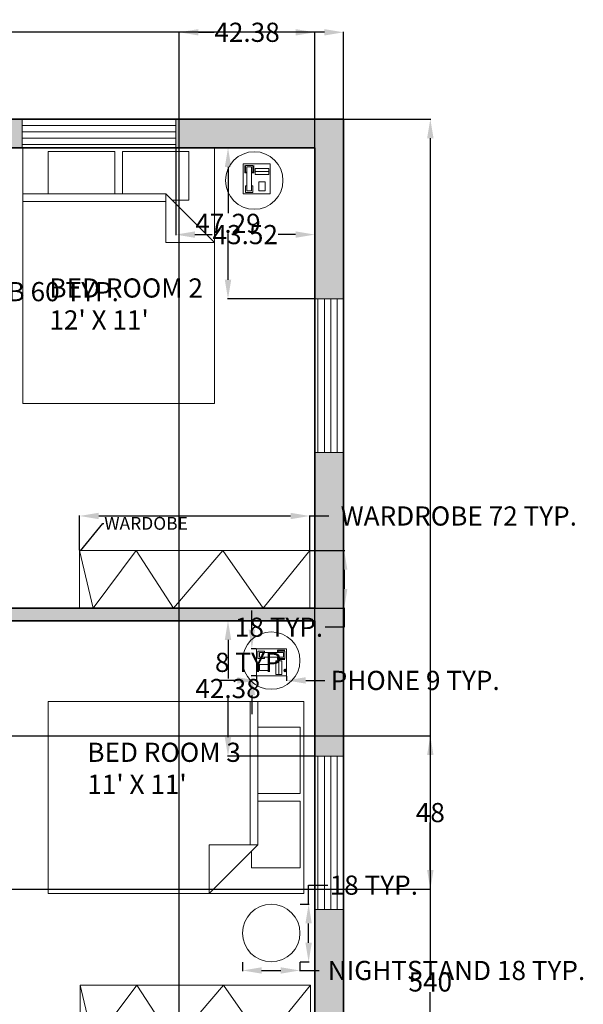
# Model space of a CAD drawing. Units: inches. Extents: x -16 to 578, y -553 to 49.
# Tile 5 of 5: x 402 to 578, y -259 to 49. Entities that reach past the tile are written whole.
import ezdxf
from ezdxf import colors
from ezdxf.entities.mleader import LeaderData, LeaderLine
from ezdxf.math import Vec2, Vec3

# ---------------------------------------------------------------- set-up
doc = ezdxf.new("R2010")
doc.units = ezdxf.units.IN
doc.header["$MEASUREMENT"] = 0
for name, color, linetype, lineweight in [('A-ANNO-DIMS', 2, 'Continuous', 18), ('A-ANNO-TEXT', 7, 'Continuous', 18), ('A-AREA-IDEN', 7, 'Continuous', 25), ('A-EQPM', 8, 'Continuous', 18), ('A-FLOR-CASE', 8, 'Continuous', 18), ('A-FURN', 8, 'Continuous', 18), ('A-GLAZ', 4, 'Continuous', 18), ('A-WALL', 7, 'Continuous', 35)]:
    doc.layers.add(name, color=color, linetype=linetype, lineweight=lineweight)
doc.layers.add('A-WALL-PATT', color=251, linetype='Continuous', lineweight=13, true_color=0x636466)
doc.styles.get("Standard").update_dxf_attribs({"font": 'arial.ttf'})
doc.dimstyles.get("Standard").update_dxf_attribs({"dimtxt": 6, "dimasz": 6, "dimexe": 0.18, "dimexo": 0.0625, "dimgap": 0.09, "dimtad": 0, "dimtih": 1, "dimtoh": 1, "dimdec": 0, "dimzin": 0, "dimdsep": 46, "dimlunit": 4, "dimtxsty": 'Standard', "dimcen": 0.09, "dimadec": 0, "dimazin": 0, "dimtfac": 1, "dimtdec": 0, "dimtofl": 0, "dimtmove": 0, "dimatfit": 3, "dimfxl": 1, "dimtolj": 1, "dimtzin": 0, "dimarcsym": 0})

# ---------------------------------------------------------------- blocks, each defined once
blk = doc.blocks.new('Bed - Queen')
for p, q in [((0, -80.00003), (0, 0)), ((0, 0), (59.99999, 0)), ((59.99999, 0), (59.99999, -80.00003)), ((7.99999, -1.2), (28.79998, -1.2)), ((7.99999, -14.4), (7.99999, -1.2)), ((28.79998, -1.2), (28.79998, -14.4)), ((31.19999, -1.2), (51.99999, -1.2)), ((31.19999, -14.4), (31.19999, -1.2)), ((51.99999, -1.2), (51.99999, -16.4)), ((0, -14.4), (44.8, -14.4)), ((59.99999, -29.6), (44.8, -14.4)), ((44.8, -14.4), (44.8, -29.6)), ((44.8, -16.8), (0, -16.8)), ((51.99999, -16.4), (46.79936, -16.4)), ((44.8, -29.6), (59.99999, -29.6)), ((59.99999, -80.00003), (0, -80.00003))]:
    blk.add_line(p, q)
blk = doc.blocks.new('Phone - Desk')
for p, q in [((-4.5, -5), (-4.5, 5)), ((-4.5, 5), (4.5, 5)), ((-4, 4.5), (-4, 2)), ((-3.75, 4.5), (-3.75, 2.25)), ((-1.25, 4.5), (-3.75, 4.5)), ((-3.25, 4), (-3.25, -4)), ((-3.25, 4), (-1.75, 4)), ((-1.75, -4), (-1.75, 4)), ((-1.25, 2.25), (-1.25, 4.5)), ((-1, 2), (-1, 4.5)), ((4, 3.5), (-0.5, 3.5)), ((-0.5, 3.5), (-0.5, 1.5)), ((4, 1.5), (4, 3.5)), ((4.5, 5), (4.5, -5)), ((-4, 2), (-3.25, 2)), ((-3.75, 2.25), (-3.25, 2.25)), ((-1.75, 2.25), (-1.25, 2.25)), ((-1.75, 2), (-1, 2)), ((-0.5, 2.5), (4, 2.5)), ((-0.5, 1.5), (4, 1.5)), ((-3.75, -2.25), (-3.25, -2.25)), ((-3.75, -4.5), (-3.75, -2.25)), ((-1.75, -2.25), (-1.25, -2.25)), ((-1.25, -2.25), (-1.25, -4.5)), ((2.75, -1), (0.75, -1)), ((0.75, -1), (0.75, -4)), ((2.75, -4), (2.75, -1)), ((4.5, -5), (-4.5, -5)), ((-1.25, -4.5), (-3.75, -4.5)), ((-3.25, -4), (-1.75, -4)), ((0.75, -4), (2.75, -4))]:
    blk.add_line(p, q)
blk = doc.blocks.new('WIN-48X9')
for p, q in [((-48, -4), (0, -4)), ((-48, -6), (0, -6)), ((-48, -8), (0, -8))]:
    blk.add_line(p, q)
for points in [[(0, 0), (0, -9), (-48, -9), (-48, 0)], [(-48, -2), (0, -2)]]:
    blk.add_lwpolyline(points, close=True)
blk = doc.blocks.new('WARDROBE-72X18')
for p, q in [((0, 0), (18, -14.58)), ((18, -14.58), (0, -27.16)), ((0, -27.16), (18, -42.59)), ((18, -42.59), (0, -54.31)), ((0, -54.31), (18, -67.75)), ((18, -67.75), (0, -72))]:
    blk.add_line(p, q)
blk.add_lwpolyline([(0, 0), (18, 0), (18, -72), (0, -72)], close=True)
blk = doc.blocks.new('NIGHTSTAND-ROUND-18')
blk.add_circle((0, 0), 9)
blk = doc.blocks.new('*D28')
at = {"layer": 'A-ANNO-DIMS', "color": 0, "lineweight": -2, "transparency": 16777216}
for p, q in [((471.56, -245.54), (471.56, -248.36)), ((489.56, -245.54), (489.56, -248.36)), ((477.56, -248.18), (483.56, -248.18)), ((489.56, -248.18), (495.56, -248.18))]:
    blk.add_line(p, q, dxfattribs=at)
at = {"layer": 'A-ANNO-DIMS', "color": 0, "transparency": 16777216}
for points in [[(477.56, -247.18), (477.56, -249.18), (471.56, -248.18)], [(483.56, -247.18), (483.56, -249.18), (489.56, -248.18)]]:
    blk.add_solid(points, dxfattribs=at)
at = {"layer": 'Defpoints', "color": 0, "transparency": 16777216}
for p in [(471.56, -245.48), (489.56, -245.48), (489.56, -248.18)]:
    blk.add_point(p, dxfattribs=at)
at = {"layer": 'A-ANNO-DIMS', "color": 0, "transparency": 16777216, "insert": (538.51, -248.18), "char_height": 6, "attachment_point": 5}
blk.add_mtext('\\A1;NIGHTSTAND 18 TYP.', dxfattribs=at)
blk = doc.blocks.new('*D29')
at = {"layer": 'A-ANNO-DIMS', "color": 0, "lineweight": -2, "transparency": 16777216}
for p, q in [((492.26, -227.48), (492.26, -221.48)), ((492.26, -221.48), (498.26, -221.48)), ((489.62, -227.48), (492.44, -227.48)), ((492.26, -239.48), (492.26, -233.48)), ((489.62, -245.48), (492.44, -245.48))]:
    blk.add_line(p, q, dxfattribs=at)
at = {"layer": 'A-ANNO-DIMS', "color": 0, "transparency": 16777216}
for points in [[(491.26, -233.48), (493.26, -233.48), (492.26, -227.48)], [(491.26, -239.48), (493.26, -239.48), (492.26, -245.48)]]:
    blk.add_solid(points, dxfattribs=at)
at = {"layer": 'Defpoints', "color": 0, "transparency": 16777216}
for p in [(489.56, -227.48), (492.26, -227.48), (489.56, -245.48)]:
    blk.add_point(p, dxfattribs=at)
at = {"layer": 'A-ANNO-DIMS', "color": 0, "transparency": 16777216, "insert": (512.67, -221.48), "char_height": 6, "attachment_point": 5}
blk.add_mtext('\\A1;18 TYP.', dxfattribs=at)
blk = doc.blocks.new('*D30')
at = {"layer": 'A-ANNO-DIMS', "color": 0, "lineweight": -2, "transparency": 16777216}
for p, q in [((420.6, -116.7), (420.6, -105.79)), ((426.6, -105.97), (486.6, -105.97)), ((492.6, -116.7), (492.6, -105.79)), ((492.6, -105.97), (498.6, -105.97))]:
    blk.add_line(p, q, dxfattribs=at)
at = {"layer": 'A-ANNO-DIMS', "color": 0, "transparency": 16777216}
for points in [[(426.6, -104.97), (426.6, -106.97), (420.6, -105.97)], [(486.6, -104.97), (486.6, -106.97), (492.6, -105.97)]]:
    blk.add_solid(points, dxfattribs=at)
at = {"layer": 'Defpoints', "color": 0, "transparency": 16777216}
for p in [(492.6, -105.97), (420.6, -116.77), (492.6, -116.77)]:
    blk.add_point(p, dxfattribs=at)
at = {"layer": 'A-ANNO-DIMS', "color": 0, "transparency": 16777216, "insert": (539.26, -105.97), "char_height": 6, "attachment_point": 5}
blk.add_mtext('\\A1;WARDROBE 72 TYP.', dxfattribs=at)
blk = doc.blocks.new('*D31')
at = {"layer": 'A-ANNO-DIMS', "color": 0, "lineweight": -2, "transparency": 16777216}
for p, q in [((492.66, -116.77), (503.58, -116.77)), ((503.4, -122.77), (503.4, -128.77)), ((492.66, -134.77), (503.58, -134.77)), ((503.4, -134.77), (503.4, -140.77)), ((503.4, -140.77), (497.4, -140.77))]:
    blk.add_line(p, q, dxfattribs=at)
at = {"layer": 'A-ANNO-DIMS', "color": 0, "transparency": 16777216}
for points in [[(502.4, -122.77), (504.4, -122.77), (503.4, -116.77)], [(502.4, -128.77), (504.4, -128.77), (503.4, -134.77)]]:
    blk.add_solid(points, dxfattribs=at)
at = {"layer": 'Defpoints', "color": 0, "transparency": 16777216}
for p in [(492.6, -116.77), (492.6, -134.77), (503.4, -134.77)]:
    blk.add_point(p, dxfattribs=at)
at = {"layer": 'A-ANNO-DIMS', "color": 0, "transparency": 16777216, "insert": (482.99, -140.77), "char_height": 6, "attachment_point": 5}
blk.add_mtext('\\A1;18 TYP.', dxfattribs=at)
blk = doc.blocks.new('*D34')
at = {"layer": 'A-ANNO-DIMS', "color": 0, "lineweight": -2, "transparency": 16777216}
for p, q in [((475.91, -156.07), (475.91, -157.6)), ((485.34, -156.07), (485.34, -157.6)), ((469.91, -157.42), (463.91, -157.42)), ((491.34, -157.42), (497.34, -157.42))]:
    blk.add_line(p, q, dxfattribs=at)
at = {"layer": 'A-ANNO-DIMS', "color": 0, "transparency": 16777216}
for points in [[(469.91, -156.42), (469.91, -158.42), (475.91, -157.42)], [(491.34, -156.42), (491.34, -158.42), (485.34, -157.42)]]:
    blk.add_solid(points, dxfattribs=at)
at = {"layer": 'Defpoints', "color": 0, "transparency": 16777216}
for p in [(475.91, -156.01), (485.34, -156.01), (485.34, -157.42)]:
    blk.add_point(p, dxfattribs=at)
at = {"layer": 'A-ANNO-DIMS', "color": 0, "transparency": 16777216, "insert": (525.62, -157.42), "char_height": 6, "attachment_point": 5}
blk.add_mtext('\\A1;PHONE 9 TYP.', dxfattribs=at)
blk = doc.blocks.new('*D35')
at = {"layer": 'A-ANNO-DIMS', "color": 0, "lineweight": -2, "transparency": 16777216}
for p, q in [((474.5, -141.53), (474.5, -135.53)), ((475.85, -147.53), (474.32, -147.53)), ((475.85, -156.01), (474.32, -156.01)), ((474.5, -162.01), (474.5, -168.01))]:
    blk.add_line(p, q, dxfattribs=at)
at = {"layer": 'A-ANNO-DIMS', "color": 0, "transparency": 16777216}
for points in [[(473.5, -141.53), (475.5, -141.53), (474.5, -147.53)], [(473.5, -162.01), (475.5, -162.01), (474.5, -156.01)]]:
    blk.add_solid(points, dxfattribs=at)
at = {"layer": 'Defpoints', "color": 0, "transparency": 16777216}
for p in [(475.91, -147.53), (474.5, -156.01), (475.91, -156.01)]:
    blk.add_point(p, dxfattribs=at)
at = {"layer": 'A-ANNO-DIMS', "color": 0, "transparency": 16777216, "insert": (474.5, -151.77), "char_height": 6, "attachment_point": 5}
blk.add_mtext('\\A1;8 TYP.', dxfattribs=at)
blk = doc.blocks.new('*D40')
at = {"layer": 'A-ANNO-DIMS', "color": 0, "lineweight": -2, "transparency": 16777216}
for p, q in [((298.19, -26.83), (298.19, -35.95)), ((358.19, -26.83), (358.19, -35.95)), ((304.19, -35.77), (352.19, -35.77)), ((358.19, -35.77), (364.19, -35.77))]:
    blk.add_line(p, q, dxfattribs=at)
at = {"layer": 'A-ANNO-DIMS', "color": 0, "transparency": 16777216}
for points in [[(304.19, -34.77), (304.19, -36.77), (298.19, -35.77)], [(352.19, -34.77), (352.19, -36.77), (358.19, -35.77)]]:
    blk.add_solid(points, dxfattribs=at)
at = {"layer": 'Defpoints', "color": 0, "transparency": 16777216}
for p in [(298.19, -26.77), (358.19, -26.77), (358.19, -35.77)]:
    blk.add_point(p, dxfattribs=at)
at = {"layer": 'A-ANNO-DIMS', "color": 0, "transparency": 16777216, "insert": (399.47, -35.77), "char_height": 6, "attachment_point": 5}
blk.add_mtext('\\A1;BATHTUB 60 TYP.', dxfattribs=at)
blk = doc.blocks.new('*D62')
at = {"layer": 'A-ANNO-DIMS', "color": 0, "lineweight": -2, "transparency": 16777216}
for p, q in [((23.19, 18.3), (23.19, 45.56)), ((29.19, 45.38), (256.36, 45.38)), ((497.19, 45.38), (270.02, 45.38)), ((503.19, 18.3), (503.19, 45.56))]:
    blk.add_line(p, q, dxfattribs=at)
at = {"layer": 'A-ANNO-DIMS', "color": 0, "transparency": 16777216}
for points in [[(29.19, 46.38), (29.19, 44.38), (23.19, 45.38)], [(497.19, 46.38), (497.19, 44.38), (503.19, 45.38)]]:
    blk.add_solid(points, dxfattribs=at)
at = {"layer": 'Defpoints', "color": 0, "transparency": 16777216}
for p in [(503.19, 45.38), (23.19, 18.23), (503.19, 18.23)]:
    blk.add_point(p, dxfattribs=at)
at = {"layer": 'A-ANNO-DIMS', "color": 0, "transparency": 16777216, "insert": (263.19, 45.38), "char_height": 6, "attachment_point": 5}
blk.add_mtext('\\A1;480', dxfattribs=at)
blk = doc.blocks.new('*D63')
at = {"layer": 'A-ANNO-DIMS', "color": 0, "lineweight": -2, "transparency": 16777216}
for p, q in [((503.25, 18.23), (530.52, 18.23)), ((530.34, 12.23), (530.34, -248.61)), ((530.34, -515.77), (530.34, -254.92)), ((503.25, -521.77), (530.52, -521.77))]:
    blk.add_line(p, q, dxfattribs=at)
at = {"layer": 'A-ANNO-DIMS', "color": 0, "transparency": 16777216}
for points in [[(529.34, 12.23), (531.34, 12.23), (530.34, 18.23)], [(529.34, -515.77), (531.34, -515.77), (530.34, -521.77)]]:
    blk.add_solid(points, dxfattribs=at)
at = {"layer": 'Defpoints', "color": 0, "transparency": 16777216}
for p in [(503.19, 18.23), (503.19, -521.77), (530.34, -521.77)]:
    blk.add_point(p, dxfattribs=at)
at = {"layer": 'A-ANNO-DIMS', "color": 0, "transparency": 16777216, "insert": (530.34, -251.77), "char_height": 6, "attachment_point": 5}
blk.add_mtext('\\A1;540', dxfattribs=at)
blk = doc.blocks.new('*D69')
at = {"layer": 'A-ANNO-DIMS', "color": 0, "lineweight": -2, "transparency": 16777216}
for p, q in [((168.25, -174.77), (530.52, -174.77)), ((530.34, -180.77), (530.34, -195.61)), ((530.34, -216.77), (530.34, -201.92)), ((168.25, -222.77), (530.52, -222.77))]:
    blk.add_line(p, q, dxfattribs=at)
at = {"layer": 'A-ANNO-DIMS', "color": 0, "transparency": 16777216}
for points in [[(529.34, -180.77), (531.34, -180.77), (530.34, -174.77)], [(529.34, -216.77), (531.34, -216.77), (530.34, -222.77)]]:
    blk.add_solid(points, dxfattribs=at)
at = {"layer": 'Defpoints', "color": 0, "transparency": 16777216}
for p in [(168.19, -174.77), (168.19, -222.77), (530.34, -222.77)]:
    blk.add_point(p, dxfattribs=at)
at = {"layer": 'A-ANNO-DIMS', "color": 0, "transparency": 16777216, "insert": (530.34, -198.77), "char_height": 6, "attachment_point": 5}
blk.add_mtext('\\A1;48', dxfattribs=at)
blk = doc.blocks.new('*D74')
at = {"layer": 'A-ANNO-DIMS', "color": 0, "lineweight": -2, "transparency": 16777216}
for p, q in [((450.67, 9.17), (450.67, -18.1)), ((494.19, 9.17), (494.19, -18.1)), ((456.67, -17.92), (462.13, -17.92)), ((488.19, -17.92), (482.73, -17.92))]:
    blk.add_line(p, q, dxfattribs=at)
at = {"layer": 'A-ANNO-DIMS', "color": 0, "transparency": 16777216}
for points in [[(456.67, -16.92), (456.67, -18.92), (450.67, -17.92)], [(488.19, -16.92), (488.19, -18.92), (494.19, -17.92)]]:
    blk.add_solid(points, dxfattribs=at)
at = {"layer": 'Defpoints', "color": 0, "transparency": 16777216}
for p in [(450.67, 9.23), (494.19, 9.23), (450.67, -17.92)]:
    blk.add_point(p, dxfattribs=at)
at = {"layer": 'A-ANNO-DIMS', "color": 0, "transparency": 16777216, "insert": (472.43, -17.92), "char_height": 6, "attachment_point": 5}
blk.add_mtext('\\A1;43.52', dxfattribs=at)
blk = doc.blocks.new('*D75')
at = {"layer": 'A-ANNO-DIMS', "color": 0, "lineweight": -2, "transparency": 16777216}
for p, q in [((494.13, 9.23), (466.86, 9.23)), ((467.04, 3.23), (467.04, -11.26)), ((467.04, -32.05), (467.04, -17.56)), ((494.13, -38.05), (466.86, -38.05))]:
    blk.add_line(p, q, dxfattribs=at)
at = {"layer": 'A-ANNO-DIMS', "color": 0, "transparency": 16777216}
for points in [[(466.04, 3.23), (468.04, 3.23), (467.04, 9.23)], [(466.04, -32.05), (468.04, -32.05), (467.04, -38.05)]]:
    blk.add_solid(points, dxfattribs=at)
at = {"layer": 'Defpoints', "color": 0, "transparency": 16777216}
for p in [(467.04, 9.23), (494.19, 9.23), (494.19, -38.05)]:
    blk.add_point(p, dxfattribs=at)
at = {"layer": 'A-ANNO-DIMS', "color": 0, "transparency": 16777216, "insert": (467.04, -14.41), "char_height": 6, "attachment_point": 5}
blk.add_mtext('\\A1;47.29', dxfattribs=at)
blk = doc.blocks.new('*D76')
at = {"layer": 'A-ANNO-DIMS', "color": 0, "lineweight": -2, "transparency": 16777216}
for p, q in [((494.13, -138.77), (466.86, -138.77)), ((467.04, -144.77), (467.04, -156.8)), ((467.04, -175.15), (467.04, -163.11)), ((494.13, -181.15), (466.86, -181.15))]:
    blk.add_line(p, q, dxfattribs=at)
at = {"layer": 'A-ANNO-DIMS', "color": 0, "transparency": 16777216}
for points in [[(466.04, -144.77), (468.04, -144.77), (467.04, -138.77)], [(466.04, -175.15), (468.04, -175.15), (467.04, -181.15)]]:
    blk.add_solid(points, dxfattribs=at)
at = {"layer": 'Defpoints', "color": 0, "transparency": 16777216}
for p in [(467.04, -138.77), (494.19, -138.77), (494.19, -181.15)]:
    blk.add_point(p, dxfattribs=at)
at = {"layer": 'A-ANNO-DIMS', "color": 0, "transparency": 16777216, "insert": (467.04, -159.96), "char_height": 6, "attachment_point": 5}
blk.add_mtext('\\A1;42.38', dxfattribs=at)
blk = doc.blocks.new('*D80')
at = {"layer": 'A-ANNO-DIMS', "color": 0, "lineweight": -2, "transparency": 16777216}
for p, q in [((451.8, -512.7), (451.8, 45.56)), ((457.8, 45.38), (462.66, 45.38)), ((488.19, 45.38), (483.34, 45.38)), ((494.19, -512.7), (494.19, 45.56))]:
    blk.add_line(p, q, dxfattribs=at)
at = {"layer": 'A-ANNO-DIMS', "color": 0, "transparency": 16777216}
for points in [[(457.8, 46.38), (457.8, 44.38), (451.8, 45.38)], [(488.19, 46.38), (488.19, 44.38), (494.19, 45.38)]]:
    blk.add_solid(points, dxfattribs=at)
at = {"layer": 'Defpoints', "color": 0, "transparency": 16777216}
for p in [(451.8, 45.38), (451.8, -512.77), (494.19, -512.77)]:
    blk.add_point(p, dxfattribs=at)
at = {"layer": 'A-ANNO-DIMS', "color": 0, "transparency": 16777216, "insert": (473, 45.38), "char_height": 6, "attachment_point": 5}
blk.add_mtext('\\A1;42.38', dxfattribs=at)

msp = doc.modelspace()

# ---------------------------------------------------------------- hatches: boundary and pattern name
at = {"layer": 'A-WALL-PATT'}
h = msp.add_hatch(color=256, dxfattribs=at)
h.dxf.hatch_style = 1
h.paths.add_polyline_path([(32.1882, 9.2337), (89.8211, 9.2337), (89.8211, 18.2337), (23.1882, 18.2337), (23.1882, -55.5259), (32.1882, -55.5259)])
h.paths.add_polyline_path([(219.6411, 18.2337), (137.8211, 18.2337), (137.8211, 9.2337), (146.4179, 9.2337), (188.1882, 9.2337), (188.1882, -98.7663), (192.1882, -98.7663), (192.1882, -72.7663), (238.1882, -72.7663), (238.1882, -68.7663), (192.1882, -68.7663), (192.1882, 9.2337), (219.6411, 9.2337)])
h.paths.add_polyline_path([(307.3924, 18.2337), (243.6411, 18.2337), (243.6411, 9.2337), (274.1882, 9.2337), (274.1882, -26.7663), (274.1882, -68.7663), (268.1882, -68.7663), (268.1882, -72.7663), (274.1882, -72.7663), (274.1882, -98.7663), (250.1882, -98.7663), (250.1882, -102.7663), (274.1882, -102.7663), (278.1882, -102.7663), (302.188, -102.8481), (302.188, -98.8481), (278.1882, -98.7663), (278.1882, -86.8559, -0.01827889), (278.1882, -85.7663), (278.1882, -72.7663), (284.1882, -72.7663), (284.1882, -68.7663), (278.1882, -68.7663), (278.1882, 9.2337), (307.3924, 9.2337)])
h.paths.add_polyline_path([(402.6701, 18.2337), (331.3924, 18.2337), (331.3924, 9.2337), (358.1882, 9.2337), (358.1882, -26.7663), (358.1882, -68.7663), (314.1882, -68.7663), (314.1882, -72.7663), (358.1882, -72.7663), (358.1882, -98.7663), (362.1882, -98.7663), (362.1882, 9.2337), (402.6701, 9.2337)])
h.paths.add_polyline_path([(503.1882, 18.2337), (450.6701, 18.2337), (450.6701, 9.2337), (462.8072, 9.2337), (494.1882, 9.2337), (494.1882, -38.053), (503.1882, -38.053)])
h.paths.add_polyline_path([(503.1882, -86.053), (494.1882, -86.053), (494.1882, -134.7663), (362.1882, -134.7663), (362.1882, -128.7663), (358.1882, -128.7663), (358.1882, -138.7663), (358.1882, -234.7663), (362.1882, -234.7663), (362.1882, -138.7663), (494.1882, -138.7663), (494.1882, -181.1501), (503.1882, -181.1501)])
h.paths.add_polyline_path([(503.1882, -229.1501), (494.1882, -229.1501), (494.1882, -270.7663), (362.1882, -270.7663), (362.1882, -264.7663), (358.1882, -264.7663), (358.1882, -294.7663), (358.1882, -323.1753), (362.1882, -323.1753), (362.1882, -298.7663), (362.1882, -294.7663), (362.1882, -274.7663), (494.1882, -274.7663), (494.1882, -294.7663), (494.1882, -298.7663), (494.1882, -310.411), (503.1882, -310.411)])
h.paths.add_polyline_path([(503.1882, -358.411), (494.1882, -358.411), (494.1882, -394.7663), (362.1882, -394.7663), (362.1882, -353.1753), (358.1882, -353.1753), (358.1882, -398.7663), (494.1882, -398.7663), (494.1882, -512.7663), (451.8049, -512.7663), (451.8049, -521.7663), (503.1882, -521.7663)])
h.paths.add_polyline_path([(403.8049, -512.7663), (176.1882, -512.7663), (176.1882, -441.7663), (172.1882, -441.7663), (172.1882, -512.7663), (150.1882, -512.7663), (150.1882, -521.7663), (403.8049, -521.7663)])
h.paths.add_polyline_path([(176.1882, -258.7663), (168.1882, -258.7663), (168.1882, -246.7663), (168.1882, -234.7663), (168.1882, -222.7663), (164.1882, -222.7663), (164.1882, -234.7663), (164.1882, -258.7663), (102.0641, -258.7663), (102.0641, -262.7663), (168.1882, -262.7663), (172.1882, -262.7663), (172.1882, -333.7663), (176.1882, -333.7663), (176.1882, -262.7663)])
h.paths.add_polyline_path([(32.1882, -262.7663), (54.0641, -262.7663), (54.0641, -258.7663), (32.1882, -258.7663), (32.1882, -229.1501), (23.1882, -229.1501), (23.1882, -283.4909), (23.1882, -470.2771), (32.1882, -470.2771), (32.1882, -283.4909)])
h.paths.add_polyline_path([(32.1882, -103.5259), (23.1882, -103.5259), (23.1882, -181.1501), (32.1882, -181.1501)])
h.paths.add_polyline_path([(192.1882, -128.7663), (188.1882, -128.7663), (188.1882, -134.7663), (32.1882, -134.7663), (32.1882, -138.7663), (164.1882, -138.7663), (164.1882, -162.7663), (164.1882, -174.7663), (168.1882, -174.7663), (168.1882, -162.7663), (168.1882, -138.7663), (192.1882, -138.7663)])

# ---------------------------------------------------------------- linework, layer by layer
at = {"layer": 'A-WALL'}
for p, q in [((362.1882, 9.2337), (494.1882, 9.2337)), ((494.1882, 9.2337), (494.1882, -134.7663)), ((362.1882, -134.7663), (494.1882, -134.7663)), ((362.1882, -138.7663), (494.1882, -138.7663)), ((494.1882, -138.7663), (494.1882, -270.7663))]:
    msp.add_line(p, q, dxfattribs=at)
msp.add_lwpolyline([(23.1882, -283.4909), (23.1882, 18.2337), (503.1882, 18.2337), (503.1882, -521.7663), (150.1882, -521.7663)], dxfattribs=at)

# ---------------------------------------------------------------- block references
at = {"layer": 'A-EQPM', "xscale": 0.9424999999999881, "yscale": 0.9424999999999881, "zscale": 0.9424999999999881}
msp.add_blockref('Phone - Desk', (476.0241, -0.4929), dxfattribs=at)
at = {"layer": 'A-EQPM', "xscale": 0.9424999999999881, "yscale": 0.9424999999999881, "zscale": 0.9424999999999881, "rotation": 270}
msp.add_blockref('Phone - Desk', (480.6266, -151.7679), dxfattribs=at)
at = {"layer": 'A-FLOR-CASE'}
for p, rotation in [((492.5998, -116.7663), 270), ((492.8002, -252.7663), 270.0000000000002)]:
    msp.add_blockref('WARDROBE-72X18', p, dxfattribs=dict(at, rotation=rotation))
at = {"layer": 'A-FURN'}
for name, p in [('Bed - Queen', (402.8072, 9.2337)), ('NIGHTSTAND-ROUND-18', (475.2432, -0.9972)), ('NIGHTSTAND-ROUND-18', (480.5554, -151.2068)), ('NIGHTSTAND-ROUND-18', (480.5554, -236.4807))]:
    msp.add_blockref(name, p, dxfattribs=at)
at = {"layer": 'A-FURN', "rotation": 270}
msp.add_blockref('Bed - Queen', (490.7863, -164.0447), dxfattribs=at)
at = {"layer": 'A-GLAZ'}
msp.add_blockref('WIN-48X9', (450.6701, 18.2337), dxfattribs=at)
for p, rotation in [((503.1882, -86.053), 270.0000000000001), ((503.1882, -229.1501), 270.0000000000002)]:
    msp.add_blockref('WIN-48X9', p, dxfattribs=dict(at, rotation=rotation))

# ---------------------------------------------------------------- texts
at = {"layer": 'A-AREA-IDEN', "char_height": 6, "attachment_point": 1}
for s, width, insert in [("BED ROOM 2\\P12' X 11'", 72.589877, (411.1588, -31.6281)), ("BED ROOM 3\\P11' X 11'", 82.456452, (423.0299, -176.9071))]:
    msp.add_mtext_dynamic_manual_height_columns(s, width=width, gutter_width=1, heights=[0], dxfattribs=dict(at, insert=insert))

# ---------------------------------------------------------------- dimensions: what is measured, and where the dimension line sits
at = {"layer": 'A-ANNO-DIMS'}
for base, p1, p2, override, picture, middle in [((503.1882, 45.3837), (23.1882, 18.2337), (503.1882, 18.2337), {"dimdec": 0, "dimlfac": 1, "dimrnd": 0, "dimzin": 0, "dimdsep": 46, "dimlunit": 2}, '*D62', (263.1882, 45.3837)), ((451.8049, 45.3837), (494.1882, -512.7663), (451.8049, -512.7663), {"dimdec": 2, "dimlfac": 1, "dimrnd": 0, "dimzin": 0, "dimdsep": 46, "dimlunit": 2}, '*D80', (472.9965, 45.3837))]:
    dim = msp.add_linear_dim(base=base, p1=p1, p2=p2, dimstyle='Standard', override=override, dxfattribs=at)
    dim.commit()
    dim.dimension.update_dxf_attribs({"geometry": picture, "text_midpoint": middle})
for base, p1, p2, angle, override, picture, middle in [((530.3382, -521.7663), (503.1882, 18.2337), (503.1882, -521.7663), 90, {"dimdec": 0, "dimlfac": 1, "dimrnd": 0, "dimzin": 0, "dimdsep": 46, "dimlunit": 2}, '*D63', (530.3382, -251.7663)), ((450.6701, -17.9163), (494.1882, 9.2337), (450.6701, 9.2337), 180, {"dimdec": 2, "dimlfac": 1, "dimrnd": 0, "dimzin": 0, "dimdsep": 46, "dimlunit": 2}, '*D74', (472.4291, -17.9163)), ((467.0382, 9.2337), (494.1882, -38.053), (494.1882, 9.2337), 90, {"dimdec": 2, "dimlfac": 1, "dimrnd": 0, "dimzin": 0, "dimdsep": 46, "dimlunit": 2}, '*D75', (467.0382, -14.4096)), ((467.0382, -138.7663), (494.1882, -181.1501), (494.1882, -138.7663), 90, {"dimdec": 2, "dimlfac": 1, "dimrnd": 0, "dimzin": 0, "dimdsep": 46, "dimlunit": 2}, '*D76', (467.0382, -159.9582)), ((530.3382, -222.7663), (168.1882, -174.7663), (168.1882, -222.7663), 90, {"dimdec": 0, "dimlfac": 1, "dimrnd": 0, "dimzin": 0, "dimdsep": 46, "dimlunit": 2}, '*D69', (530.3382, -198.7663))]:
    dim = msp.add_linear_dim(base=base, p1=p1, p2=p2, angle=angle, dimstyle='Standard', override=override, dxfattribs=at)
    dim.commit()
    dim.dimension.update_dxf_attribs({"geometry": picture, "text_midpoint": middle})
for base, p1, p2, text, picture, middle in [((358.1882, -35.7663), (298.1882, -26.7663), (358.1882, -26.7663), 'BATHTUB <> TYP.', '*D40', (399.4719, -35.7663)), ((492.5998, -105.9663), (420.5998, -116.7663), (492.5998, -116.7663), 'WARDROBE <> TYP.', '*D30', (539.2614, -105.9663)), ((485.3391, -157.4229), (475.9141, -156.0092), (485.3391, -156.0092), 'PHONE <> TYP.', '*D34', (525.6201, -157.4229)), ((489.5554, -248.1807), (471.5554, -245.4807), (489.5554, -245.4807), 'NIGHTSTAND <> TYP.', '*D28', (538.509, -248.1807))]:
    dim = msp.add_linear_dim(base=base, p1=p1, p2=p2, text=text, dimstyle='Standard', override={"dimdec": 0, "dimlfac": 1, "dimrnd": 0, "dimzin": 0, "dimdsep": 46, "dimlunit": 2}, dxfattribs=at)
    dim.commit()
    dim.dimension.update_dxf_attribs({"geometry": picture, "text_midpoint": middle})
for base, p1, p2, angle, picture, middle in [((503.3998, -134.7663), (492.5998, -116.7663), (492.5998, -134.7663), 270, '*D31', (482.9892, -140.7663)), ((474.5004, -156.0092), (475.9141, -147.5267), (475.9141, -156.0092), 270, '*D35', (474.5004, -151.7679)), ((492.2554, -227.4807), (489.5554, -245.4807), (489.5554, -227.4807), 90, '*D29', (512.666, -221.4807))]:
    dim = msp.add_linear_dim(base=base, p1=p1, p2=p2, angle=angle, text='<> TYP.', dimstyle='Standard', override={"dimdec": 0, "dimlfac": 1, "dimrnd": 0, "dimzin": 0, "dimdsep": 46, "dimlunit": 2}, dxfattribs=at)
    dim.commit()
    dim.dimension.update_dxf_attribs({"geometry": picture, "text_midpoint": middle})

# ---------------------------------------------------------------- leaders
at = {"layer": 'A-ANNO-TEXT'}
ml = msp.add_multileader_mtext('Standard', dxfattribs=at)
ml.set_content('WARDOBE', color=256)
ml.set_leader_properties()
ml.build(insert=Vec2(0, 0))
ml.multileader.update_dxf_attribs({"dogleg_length": 0.36, "arrow_head_size": 0})
ctx = ml.context
ctx.base_point, ctx.arrow_head_size, ctx.landing_gap_size, ctx.plane_origin = Vec3(428.2297, -108.3064), 0, 0.09, Vec3(420.8986, -116.9137)
notes = []
notes.append((ctx, [(0, (1, 1, 0), (427.8697, -108.3064), (1, 0), 0.36, [(0, [(420.8986, -116.9137)], 0, [])])]))
ctx.mtext.insert, ctx.mtext.width, ctx.mtext.flow_direction = Vec3(428.3197, -106.2722), 4, 5
for ctx, leaders in notes:
    for number, flags, end, landing, length, lines in leaders:
        leader = LeaderData()
        leader.index, (leader.has_last_leader_line, leader.has_dogleg_vector, leader.attachment_direction) = number, flags
        leader.last_leader_point, leader.dogleg_vector, leader.dogleg_length = Vec3(end), Vec3(landing), length
        for number, points, colour, breaks in lines:
            line = LeaderLine()
            line.index, line.vertices, line.color, line.breaks = number, Vec3.list(points), colors.encode_raw_color(colour), breaks
            leader.lines.append(line)
        ctx.leaders.append(leader)

doc.saveas('drawing.dxf')
